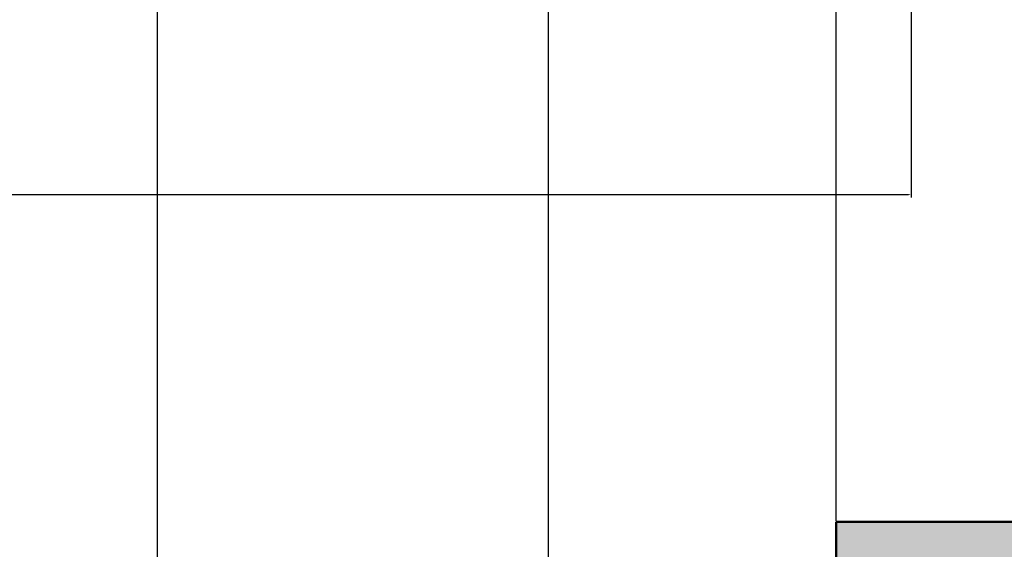
# Model space of a CAD drawing. Units: inches. Extents: x 2974 to 3443, y 2405 to 2963.
# Tile 7 of 13: x 3276 to 3341, y 2607 to 2643. Entities that reach past the tile are written whole.
import ezdxf

# ---------------------------------------------------------------- set-up
doc = ezdxf.new("R2010")
doc.units = ezdxf.units.IN
doc.header["$MEASUREMENT"] = 0
for name, color, linetype, lineweight in [('A-ANNO-DIMS', 2, 'Continuous', 18), ('A-WALL-PATT', 252, 'Continuous', 13), ('walls', 250, 'Continuous', 50)]:
    doc.layers.add(name, color=color, linetype=linetype, lineweight=lineweight)
doc.styles.get("Standard").update_dxf_attribs({"font": 'arial.ttf'})
doc.dimstyles.get("Standard").update_dxf_attribs({"dimtxt": 7, "dimasz": 0.18, "dimexe": 0.18, "dimexo": 0.0625, "dimgap": 0.09, "dimtad": 0, "dimtih": 1, "dimtoh": 1, "dimzin": 0, "dimdsep": 46, "dimlunit": 3, "dimtxsty": 'Standard', "dimcen": 0.09, "dimadec": 0, "dimazin": 0, "dimtfac": 1, "dimtofl": 0, "dimtmove": 0, "dimatfit": 3, "dimfxl": 1, "dimtolj": 1, "dimtzin": 0, "dimarcsym": 0})

# ---------------------------------------------------------------- blocks, each defined once
blk = doc.blocks.new('*D47')
at = {"layer": 'A-ANNO-DIMS', "color": 0, "lineweight": -2, "transparency": 16777216}
for p, q in [((3247.425, 2644.017), (3247.425, 2630.764)), ((3334.991, 2644.017), (3334.991, 2630.764)), ((3247.425, 2630.944), (3247.245, 2630.944)), ((3334.811, 2630.944), (3247.605, 2630.944))]:
    blk.add_line(p, q, dxfattribs=at)
at = {"layer": 'A-ANNO-DIMS', "color": 0, "transparency": 16777216}
for points in [[(3247.605, 2630.974), (3247.605, 2630.914), (3247.425, 2630.944)], [(3334.811, 2630.974), (3334.811, 2630.914), (3334.991, 2630.944)]]:
    blk.add_solid(points, dxfattribs=at)
at = {"layer": 'Defpoints', "color": 0, "transparency": 16777216}
for p in [(3247.425, 2644.079), (3334.991, 2644.079), (3247.425, 2630.944)]:
    blk.add_point(p, dxfattribs=at)
at = {"layer": 'A-ANNO-DIMS', "color": 0, "transparency": 16777216, "insert": (3200.531, 2630.944), "char_height": 7, "attachment_point": 5}
blk.add_mtext('\\A1;DINING SET 7\'-3 1/2"', dxfattribs=at)
blk = doc.blocks.new('*D62')
at = {"layer": 'A-ANNO-DIMS', "color": 0, "lineweight": -2, "transparency": 16777216}
for p, q in [((3267.326, 2609.251), (3267.326, 2952.678)), ((3267.506, 2952.498), (3281.115, 2952.498)), ((3329.823, 2952.498), (3316.214, 2952.498)), ((3330.003, 2609.251), (3330.003, 2952.678))]:
    blk.add_line(p, q, dxfattribs=at)
at = {"layer": 'A-ANNO-DIMS', "color": 0, "transparency": 16777216}
for points in [[(3267.506, 2952.528), (3267.506, 2952.468), (3267.326, 2952.498)], [(3329.823, 2952.528), (3329.823, 2952.468), (3330.003, 2952.498)]]:
    blk.add_solid(points, dxfattribs=at)
at = {"layer": 'Defpoints', "color": 0, "transparency": 16777216}
for p in [(3330.003, 2952.498), (3267.326, 2609.188), (3330.003, 2609.188)]:
    blk.add_point(p, dxfattribs=at)
at = {"layer": 'A-ANNO-DIMS', "color": 0, "transparency": 16777216, "insert": (3298.665, 2952.498), "char_height": 7, "attachment_point": 5}
blk.add_mtext('\\A1;5\'-2 1/2"', dxfattribs=at)
blk = doc.blocks.new('*D63')
at = {"layer": 'A-ANNO-DIMS', "color": 0, "lineweight": -2, "transparency": 16777216}
for p, q in [((3244.826, 2751.126), (3244.826, 2414.917)), ((3284.826, 2751.126), (3284.826, 2414.917)), ((3245.006, 2415.097), (3255.434, 2415.097)), ((3284.646, 2415.097), (3274.217, 2415.097))]:
    blk.add_line(p, q, dxfattribs=at)
at = {"layer": 'A-ANNO-DIMS', "color": 0, "transparency": 16777216}
for points in [[(3245.006, 2415.127), (3245.006, 2415.067), (3244.826, 2415.097)], [(3284.646, 2415.127), (3284.646, 2415.067), (3284.826, 2415.097)]]:
    blk.add_solid(points, dxfattribs=at)
at = {"layer": 'Defpoints', "color": 0, "transparency": 16777216}
for p in [(3244.826, 2751.188), (3284.826, 2751.188), (3284.826, 2415.097)]:
    blk.add_point(p, dxfattribs=at)
at = {"layer": 'A-ANNO-DIMS', "color": 0, "transparency": 16777216, "insert": (3264.826, 2415.097), "char_height": 7, "attachment_point": 5}
blk.add_mtext('\\A1;3\'-4"', dxfattribs=at)
blk = doc.blocks.new('*D78')
at = {"layer": 'A-ANNO-DIMS', "color": 0, "lineweight": -2, "transparency": 16777216}
for p, q in [((3267.326, 2480.251), (3267.326, 2952.678)), ((3267.506, 2952.498), (3271.548, 2952.498)), ((3310.684, 2952.498), (3306.642, 2952.498)), ((3310.864, 2481.932), (3310.864, 2952.678))]:
    blk.add_line(p, q, dxfattribs=at)
at = {"layer": 'A-ANNO-DIMS', "color": 0, "transparency": 16777216}
for points in [[(3267.506, 2952.528), (3267.506, 2952.468), (3267.326, 2952.498)], [(3310.684, 2952.528), (3310.684, 2952.468), (3310.864, 2952.498)]]:
    blk.add_solid(points, dxfattribs=at)
at = {"layer": 'Defpoints', "color": 0, "transparency": 16777216}
for p in [(3310.864, 2952.498), (3310.864, 2481.869), (3267.326, 2480.188)]:
    blk.add_point(p, dxfattribs=at)
at = {"layer": 'A-ANNO-DIMS', "color": 0, "transparency": 16777216, "insert": (3289.095, 2952.498), "char_height": 7, "attachment_point": 5}
blk.add_mtext('\\A1;3\'-7 1/2"', dxfattribs=at)

msp = doc.modelspace()

# ---------------------------------------------------------------- hatches: boundary and pattern name
at = {"layer": 'A-WALL-PATT'}
h = msp.add_hatch(color=256, dxfattribs=at)
h.dxf.hatch_style = 1
h.paths.add_polyline_path([(3222.294, 2555.188), (3211.826, 2555.188), (3211.826, 2657.938), (3207.326, 2657.938), (3207.326, 2555.188), (3051.326, 2555.188), (3051.326, 2583.943), (3042.326, 2583.943), (3042.326, 2471.188), (3165.027, 2471.188), (3165.027, 2480.188), (3051.326, 2480.188), (3051.326, 2550.688), (3222.294, 2550.688)])
h.paths.add_polyline_path([(3188.326, 2700.207), (3183.826, 2700.207), (3183.826, 2691.688), (3051.326, 2691.688), (3051.326, 2740.572), (3042.326, 2740.572), (3042.326, 2651.235), (3045.517, 2651.235), (3051.326, 2651.235), (3051.326, 2687.188), (3188.326, 2687.188)])
h.paths.add_polyline_path([(3051.326, 2894.188), (3074.298, 2894.188), (3074.298, 2903.188), (3042.326, 2903.188), (3042.326, 2807.864), (3045.517, 2807.864), (3051.326, 2807.864), (3051.326, 2835.688), (3103.457, 2835.688), (3103.457, 2839.066, -0.012473), (3103.485, 2840.188), (3051.326, 2840.188)])
h.paths.add_polyline_path([(3201.987, 2903.188), (3100.263, 2903.188), (3100.263, 2894.188), (3131.326, 2894.188), (3131.326, 2835.688), (3135.826, 2835.688), (3135.826, 2894.188), (3183.826, 2894.188), (3183.826, 2840.188), (3159.826, 2840.188), (3159.826, 2835.688), (3183.826, 2835.688), (3183.826, 2740.207), (3188.326, 2740.207), (3188.326, 2803.688), (3215.422, 2803.688), (3215.422, 2807.066, -0.012473), (3215.45, 2808.188), (3188.326, 2808.188), (3188.326, 2894.188), (3201.987, 2894.188)])
h.paths.add_polyline_path([(3283.564, 2903.188), (3227.952, 2903.188), (3227.952, 2894.188), (3240.326, 2894.188), (3240.326, 2755.688), (3188.326, 2755.688), (3188.326, 2751.188), (3244.826, 2751.188), (3244.826, 2757.188), (3244.826, 2797.188), (3244.826, 2894.188), (3283.564, 2894.188)])
h.paths.add_polyline_path([(3384.326, 2903.188), (3346.694, 2903.188), (3346.694, 2894.188), (3375.326, 2894.188), (3375.326, 2755.688), (3284.826, 2755.688), (3284.826, 2751.188), (3375.326, 2751.188), (3375.326, 2710.653), (3378.517, 2710.653), (3384.326, 2710.653)])
h.paths.add_polyline_path([(3384.326, 2643.361), (3375.326, 2643.361), (3375.326, 2609.188), (3330.003, 2609.188), (3330.003, 2604.688), (3375.326, 2604.688), (3375.326, 2480.188), (3356.49, 2480.188), (3356.49, 2471.188), (3384.326, 2471.188)])
h.paths.add_polyline_path([(3267.326, 2609.188), (3262.826, 2609.188), (3262.826, 2555.188), (3257.429, 2555.188), (3257.429, 2550.688), (3262.826, 2550.688), (3262.826, 2471.188), (3293.36, 2471.188), (3293.36, 2480.188), (3267.326, 2480.188)])
h.paths.add_polyline_path([(3275.186, 2471.188), (3268.471, 2471.188), (3268.471, 2455.229), (3268.471, 2452.413), (3275.186, 2452.413)])
h.paths.add_polyline_path([(3156.684, 2471.188), (3149.969, 2471.188), (3149.969, 2452.413), (3156.684, 2452.413)])

# ---------------------------------------------------------------- linework, layer by layer
at = {"layer": 'walls'}
for q in [(3330.003, 2604.688), (3375.326, 2609.188)]:
    msp.add_line((3330.003, 2609.188), q, dxfattribs=at)

# ---------------------------------------------------------------- dimensions: what is measured, and where the dimension line sits
at = {"layer": 'A-ANNO-DIMS'}
for base, p1, p2, picture, middle in [((3330.003, 2952.498), (3267.326, 2609.188), (3330.003, 2609.188), '*D62', (3298.665, 2952.498)), ((3310.864, 2952.498), (3267.326, 2480.188), (3310.864, 2481.869), '*D78', (3289.095, 2952.498)), ((3284.826, 2415.097), (3244.826, 2751.188), (3284.826, 2751.188), '*D63', (3264.826, 2415.097))]:
    dim = msp.add_linear_dim(base=base, p1=p1, p2=p2, dimstyle='Standard', override={"dimdec": 1, "dimlfac": 1, "dimrnd": 0, "dimzin": 1, "dimdsep": 46, "dimlunit": 4, "dimfrac": 2}, dxfattribs=at)
    dim.commit()
    dim.dimension.update_dxf_attribs({"geometry": picture, "text_midpoint": middle})
dim = msp.add_linear_dim(base=(3247.425, 2630.944), p1=(3334.991, 2644.079), p2=(3247.425, 2644.079), angle=180, text='DINING SET <>', dimstyle='Standard', override={"dimdec": 1, "dimlfac": 1, "dimrnd": 0, "dimzin": 1, "dimdsep": 46, "dimlunit": 4, "dimfrac": 2}, dxfattribs=at)
dim.commit()
dim.dimension.update_dxf_attribs({"geometry": '*D47', "text_midpoint": (3200.531, 2630.944)})

doc.saveas('drawing.dxf')
